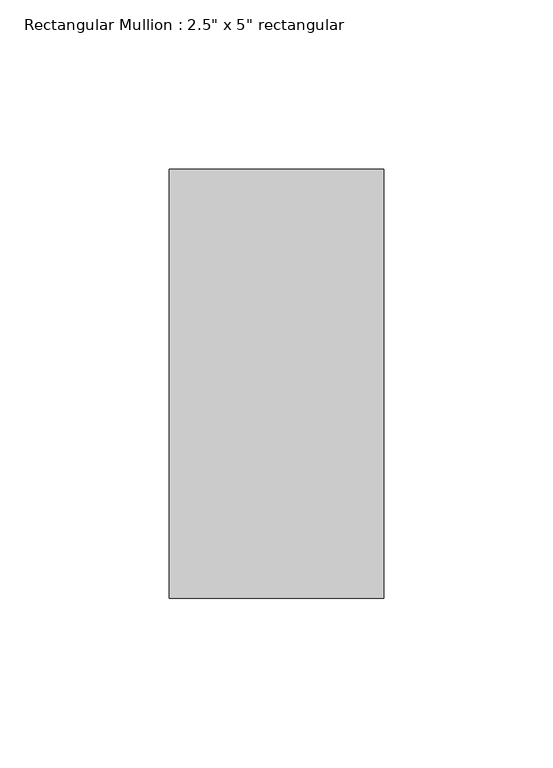
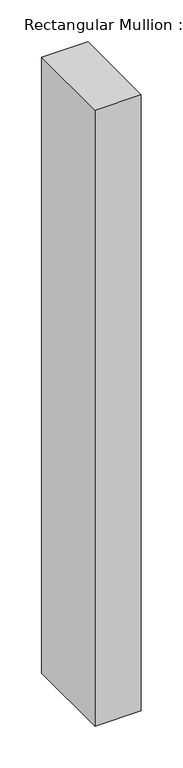
"""IFC4 building model written with IfcOpenShell, lengths in millimetres: member geometry."""

from ifc_helpers import new_model, si_unit, frame, origin, place, context, project, spatial, polyline, outline, extrude, source, transform, mapped, element, save


def member_e0487b50(model_context):
    return source(origin(), model_context, "Body", "SweptSolid", [
        extrude(outline(polyline([(31.75, 63.5), (31.75, -63.5), (-31.75, -63.5), (-31.75, 63.5), (31.75, 63.5)])), frame((0.0, 0.0, -895.35), z_axis=(0.0, 0.0, 1.0), x_axis=(1.0, 0.0, 0.0)), (0.0, 0.0, 1.0), 895.35),
    ])


if __name__ == "__main__":
    model = new_model("IFC4")
    model_context = context("Model", 3, world=origin())
    ifc_project = project(units=[si_unit("LENGTHUNIT", "METRE", prefix="MILLI")], contexts=[model_context])
    site = spatial("IfcSite", under=ifc_project)
    building = spatial("IfcBuilding", under=site)
    placement = place(None, origin())
    member_shape = member_e0487b50(model_context)
    element("IfcMember", 1, ObjectType="Rectangular Mullion : 2.5\" x 5\" rectangular", at=placement, inside=building, context=model_context, shape_type="MappedRepresentation", body=[
        mapped(member_shape, transform((0.0, 0.0, 0.0), x_axis=(1.0, 0.0, 0.0), y_axis=(0.0, 1.0, 0.0), z_axis=(0.0, 0.0, 1.0))),
    ])
    save(model, "model.ifc")

# Revit data of these elements
# Type "Rectangular Mullion : 2.5\" x 5\" rectangular"
#   built-in parameter 1007304 = 0.416667 (stored number, unit not read)
#   built-in parameter 1007301 = 0.104167 (stored number, unit not read)
#   built-in parameter 1007300 = 0.104167 (stored number, unit not read)
# Element 1 (IfcMember, "Rectangular Mullion : 2.5\" x 5\" rectangular")
#   Materials on its faces: "Aluminum"
# Materials
#   "Aluminum": class "Metal", colour RGB 247 247 247, transparency 0, Description = "Aluminum 6061", Cost = 0
